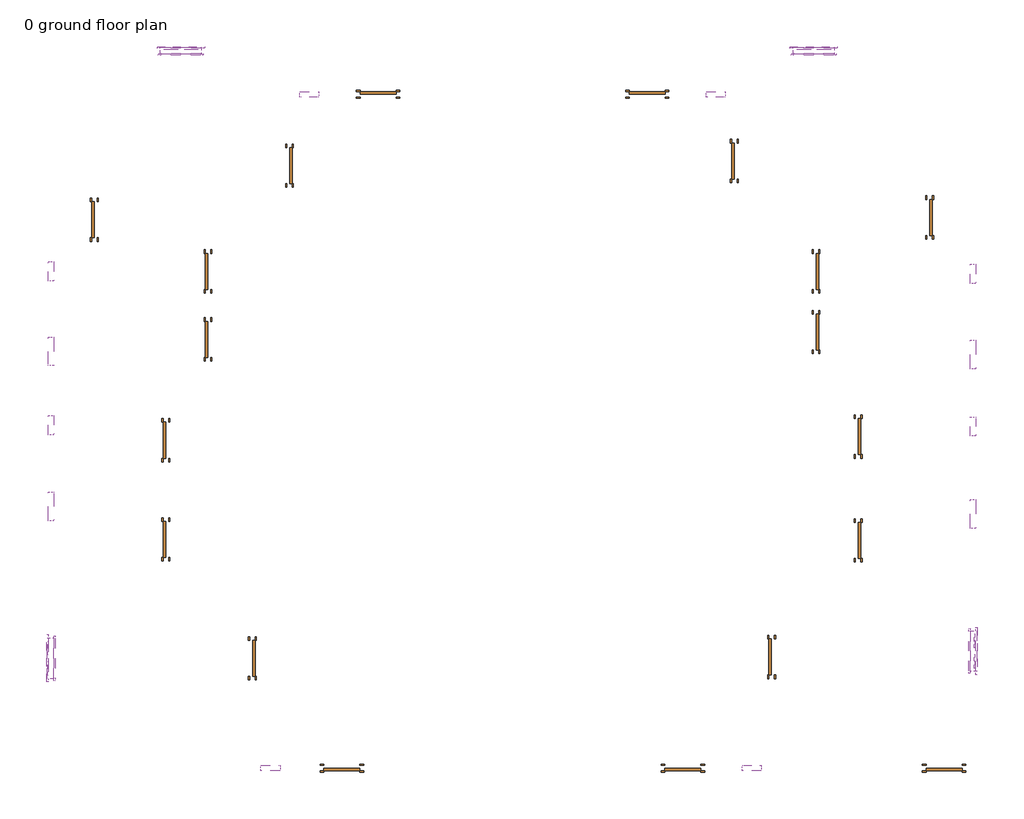
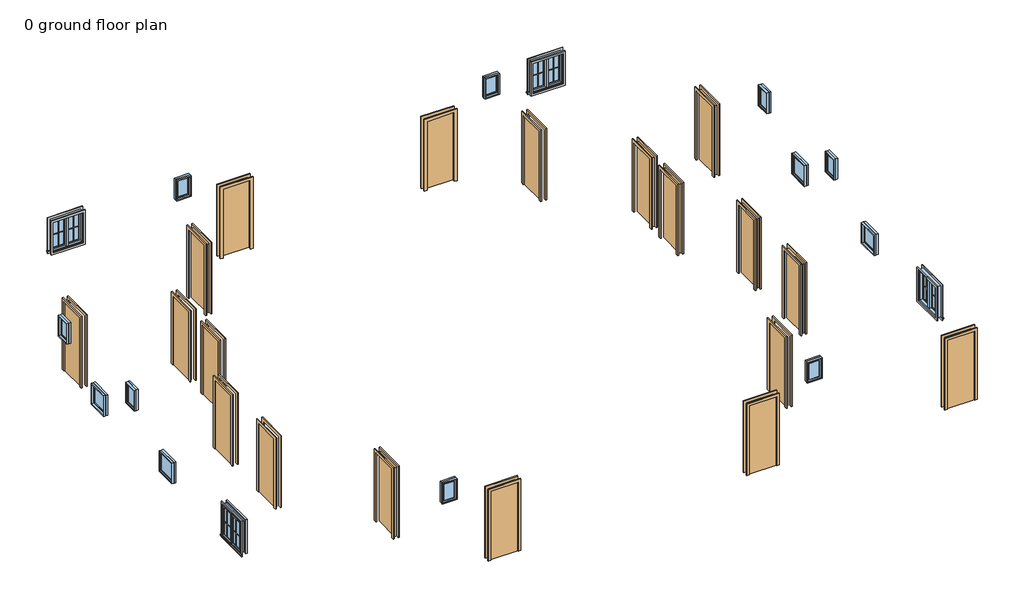
# One storey, incomplete: 19 doors, 16 proxies, 16 windows.
"""IFC4 building model written with IfcOpenShell, lengths in millimetres."""

from ifc_helpers import new_model, si_unit, origin, place, context, project, spatial, transform, mapped, element, save
from components import muntin_pattern_2x2_muntin_pattern_2x2_b3fe6957, muntin_pattern_2x2_muntin_pattern_2x2_3e0ecaf2, trim_window_exterior_flat_with_sill_41619996, trim_window_interior_flat_picture_frame_51c85655, door_f2b275c1, door_d8f5dbb5, window_a10b4202, window_0e670d86, window_a598f463

model = new_model("IFC4")

# Units and contexts
model_context = context("Model", 3, world=origin())
ifc_project = project(units=[si_unit("LENGTHUNIT", "METRE", prefix="MILLI")], contexts=[model_context])

# Site, building, storey
site = spatial("IfcSite", under=ifc_project)
building = spatial("IfcBuilding", under=site)
storey = spatial("IfcBuildingStorey", under=building, Name="0 ground floor plan", Elevation=0.0)

# Proxies
placement = place(None, origin())
muntin_pattern_2x2_muntin_pattern_2x2_shape = muntin_pattern_2x2_muntin_pattern_2x2_b3fe6957(model_context)
element("IfcBuildingElementProxy", 1, Name="Muntin Pattern_2x2 : Muntin Pattern_2x2", ObjectType="Muntin Pattern_2x2 : Muntin Pattern_2x2", at=placement, inside=storey, context=model_context, shape_type="MappedRepresentation", body=[
    mapped(muntin_pattern_2x2_muntin_pattern_2x2_shape, transform((-12267.1468188, 5178.6185601, 1593.85), x_axis=(1.0, 0.0, 0.0), y_axis=(0.0, 1.0, 0.0), z_axis=(0.0, 0.0, 1.0))),
])
element("IfcBuildingElementProxy", 2, Name="Muntin Pattern_2x2 : Muntin Pattern_2x2", ObjectType="Muntin Pattern_2x2 : Muntin Pattern_2x2", at=placement, inside=storey, context=model_context, shape_type="MappedRepresentation", body=[
    mapped(muntin_pattern_2x2_muntin_pattern_2x2_shape, transform((1105.9531812, 5178.6185601, 1593.85), x_axis=(1.0, 0.0, 0.0), y_axis=(0.0, 1.0, 0.0), z_axis=(0.0, 0.0, 1.0))),
])
element("IfcBuildingElementProxy", 3, Name="Muntin Pattern_2x2 : Muntin Pattern_2x2", ObjectType="Muntin Pattern_2x2 : Muntin Pattern_2x2", at=placement, inside=storey, context=model_context, shape_type="MappedRepresentation", body=[
    mapped(muntin_pattern_2x2_muntin_pattern_2x2_shape, transform((4733.3906812, -7341.9939399, 1593.85), x_axis=(0.0, -1.0, 0.0), y_axis=(1.0, 0.0, 0.0), z_axis=(0.0, 0.0, 1.0))),
])
element("IfcBuildingElementProxy", 4, Name="Muntin Pattern_2x2 : Muntin Pattern_2x2", ObjectType="Muntin Pattern_2x2 : Muntin Pattern_2x2", at=placement, inside=storey, context=model_context, shape_type="MappedRepresentation", body=[
    mapped(muntin_pattern_2x2_muntin_pattern_2x2_shape, transform((-14843.6593188, -7923.0189399, 1593.85), x_axis=(0.0, 1.0, 0.0), y_axis=(-1.0, 0.0, 0.0), z_axis=(0.0, 0.0, 1.0))),
])
muntin_pattern_2x2_muntin_pattern_2x2_2_shape = muntin_pattern_2x2_muntin_pattern_2x2_3e0ecaf2(model_context)
element("IfcBuildingElementProxy", 5, Name="Muntin Pattern_2x2 : Muntin Pattern_2x2", ObjectType="Muntin Pattern_2x2 : Muntin Pattern_2x2", at=placement, inside=storey, context=model_context, shape_type="MappedRepresentation", body=[
    mapped(muntin_pattern_2x2_muntin_pattern_2x2_2_shape, transform((-11838.5218188, 5178.6185601, 1593.85), x_axis=(-1.0, 0.0, 0.0), y_axis=(0.0, -1.0, 0.0), z_axis=(0.0, 0.0, 1.0))),
])
element("IfcBuildingElementProxy", 6, Name="Muntin Pattern_2x2 : Muntin Pattern_2x2", ObjectType="Muntin Pattern_2x2 : Muntin Pattern_2x2", at=placement, inside=storey, context=model_context, shape_type="MappedRepresentation", body=[
    mapped(muntin_pattern_2x2_muntin_pattern_2x2_2_shape, transform((1534.5781812, 5178.6185601, 1593.85), x_axis=(-1.0, 0.0, 0.0), y_axis=(0.0, -1.0, 0.0), z_axis=(0.0, 0.0, 1.0))),
])
element("IfcBuildingElementProxy", 7, Name="Muntin Pattern_2x2 : Muntin Pattern_2x2", ObjectType="Muntin Pattern_2x2 : Muntin Pattern_2x2", at=placement, inside=storey, context=model_context, shape_type="MappedRepresentation", body=[
    mapped(muntin_pattern_2x2_muntin_pattern_2x2_2_shape, transform((4733.3906812, -7770.6189399, 1593.85), x_axis=(0.0, 1.0, 0.0), y_axis=(-1.0, 0.0, 0.0), z_axis=(0.0, 0.0, 1.0))),
])
element("IfcBuildingElementProxy", 8, Name="Muntin Pattern_2x2 : Muntin Pattern_2x2", ObjectType="Muntin Pattern_2x2 : Muntin Pattern_2x2", at=placement, inside=storey, context=model_context, shape_type="MappedRepresentation", body=[
    mapped(muntin_pattern_2x2_muntin_pattern_2x2_2_shape, transform((-14843.6593188, -7494.3939399, 1593.85), x_axis=(0.0, -1.0, 0.0), y_axis=(1.0, 0.0, 0.0), z_axis=(0.0, 0.0, 1.0))),
])
trim_window_exterior_flat_with_sill_shape = trim_window_exterior_flat_with_sill_41619996(model_context)
element("IfcBuildingElementProxy", 9, Name="Trim-Window-Exterior-Flat : with Sill", ObjectType="Trim-Window-Exterior-Flat : with Sill", at=placement, inside=storey, context=model_context, shape_type="MappedRepresentation", body=[
    mapped(trim_window_exterior_flat_with_sill_shape, transform((-12052.8343188, 5188.1435601, 2438.4), x_axis=(-1.0, 0.0, 0.0), y_axis=(0.0, 0.0, 1.0), z_axis=(0.0, 1.0, 0.0))),
])
element("IfcBuildingElementProxy", 10, Name="Trim-Window-Exterior-Flat : with Sill", ObjectType="Trim-Window-Exterior-Flat : with Sill", at=placement, inside=storey, context=model_context, shape_type="MappedRepresentation", body=[
    mapped(trim_window_exterior_flat_with_sill_shape, transform((1320.2656812, 5188.1435601, 2438.4), x_axis=(-1.0, 0.0, 0.0), y_axis=(0.0, 0.0, 1.0), z_axis=(0.0, 1.0, 0.0))),
])
element("IfcBuildingElementProxy", 11, Name="Trim-Window-Exterior-Flat : with Sill", ObjectType="Trim-Window-Exterior-Flat : with Sill", at=placement, inside=storey, context=model_context, shape_type="MappedRepresentation", body=[
    mapped(trim_window_exterior_flat_with_sill_shape, transform((4742.9156812, -7556.3064399, 2438.4), x_axis=(0.0, 1.0, 0.0), y_axis=(0.0, 0.0, 1.0), z_axis=(1.0, 0.0, 0.0))),
])
element("IfcBuildingElementProxy", 12, Name="Trim-Window-Exterior-Flat : with Sill", ObjectType="Trim-Window-Exterior-Flat : with Sill", at=placement, inside=storey, context=model_context, shape_type="MappedRepresentation", body=[
    mapped(trim_window_exterior_flat_with_sill_shape, transform((-14853.1843188, -7708.7064399, 2438.4), x_axis=(0.0, -1.0, 0.0), y_axis=(0.0, 0.0, 1.0), z_axis=(-1.0, 0.0, 0.0))),
])
trim_window_interior_flat_picture_frame_shape = trim_window_interior_flat_picture_frame_51c85655(model_context)
element("IfcBuildingElementProxy", 13, Name="Trim-Window-Interior-Flat : Picture Frame", ObjectType="Trim-Window-Interior-Flat : Picture Frame", at=placement, inside=storey, context=model_context, shape_type="MappedRepresentation", body=[
    mapped(trim_window_interior_flat_picture_frame_shape, transform((-12052.8343188, 5073.8435601, 2438.4), x_axis=(1.0, 0.0, 0.0), y_axis=(0.0, 0.0, 1.0), z_axis=(0.0, -1.0, 0.0))),
])
element("IfcBuildingElementProxy", 14, Name="Trim-Window-Interior-Flat : Picture Frame", ObjectType="Trim-Window-Interior-Flat : Picture Frame", at=placement, inside=storey, context=model_context, shape_type="MappedRepresentation", body=[
    mapped(trim_window_interior_flat_picture_frame_shape, transform((1320.2656812, 5073.8435601, 2438.4), x_axis=(1.0, 0.0, 0.0), y_axis=(0.0, 0.0, 1.0), z_axis=(0.0, -1.0, 0.0))),
])
element("IfcBuildingElementProxy", 15, Name="Trim-Window-Interior-Flat : Picture Frame", ObjectType="Trim-Window-Interior-Flat : Picture Frame", at=placement, inside=storey, context=model_context, shape_type="MappedRepresentation", body=[
    mapped(trim_window_interior_flat_picture_frame_shape, transform((4628.6156812, -7556.3064399, 2438.4), x_axis=(0.0, -1.0, 0.0), y_axis=(0.0, 0.0, 1.0), z_axis=(-1.0, 0.0, 0.0))),
])
element("IfcBuildingElementProxy", 16, Name="Trim-Window-Interior-Flat : Picture Frame", ObjectType="Trim-Window-Interior-Flat : Picture Frame", at=placement, inside=storey, context=model_context, shape_type="MappedRepresentation", body=[
    mapped(trim_window_interior_flat_picture_frame_shape, transform((-14738.8843188, -7708.7064399, 2438.4), x_axis=(0.0, 1.0, 0.0), y_axis=(0.0, 0.0, 1.0), z_axis=(1.0, 0.0, 0.0))),
])

# Doors
door_shape = door_f2b275c1(model_context)
element("IfcDoor", 17, ObjectType="Single-Flush : 30\" x 80\"", at=placement, inside=storey, context=model_context, shape_type="MappedRepresentation", body=[
    mapped(door_shape, transform((-7885.3769874, 4216.5935601, 457.2), x_axis=(-1.0, 0.0, 0.0), y_axis=(0.0, -1.0, 0.0), z_axis=(0.0, 0.0, 1.0))),
])
element("IfcDoor", 18, ObjectType="Single-Flush : 30\" x 80\"", at=placement, inside=storey, context=model_context, shape_type="MappedRepresentation", body=[
    mapped(door_shape, transform((-13881.6343188, 1562.2935601, 457.2), x_axis=(0.0, -1.0, 0.0), y_axis=(1.0, 0.0, 0.0), z_axis=(0.0, 0.0, 1.0))),
])
element("IfcDoor", 19, ObjectType="Single-Flush : 30\" x 80\"", at=placement, inside=storey, context=model_context, shape_type="MappedRepresentation", body=[
    mapped(door_shape, transform((1371.0656812, 470.0935601, 457.2), x_axis=(0.0, 1.0, 0.0), y_axis=(-1.0, 0.0, 0.0), z_axis=(0.0, 0.0, 1.0))),
])
element("IfcDoor", 20, ObjectType="Single-Flush : 30\" x 80\"", at=placement, inside=storey, context=model_context, shape_type="MappedRepresentation", body=[
    mapped(door_shape, transform((1371.0656812, -812.6064399, 457.2), x_axis=(0.0, 1.0, 0.0), y_axis=(-1.0, 0.0, 0.0), z_axis=(0.0, 0.0, 1.0))),
])
element("IfcDoor", 21, ObjectType="Single-Flush : 30\" x 80\"", at=placement, inside=storey, context=model_context, shape_type="MappedRepresentation", body=[
    mapped(door_shape, transform((-1442.1535225, -10032.8064399, 457.2), x_axis=(1.0, 0.0, 0.0), y_axis=(0.0, 1.0, 0.0), z_axis=(0.0, 0.0, 1.0))),
])
element("IfcDoor", 22, ObjectType="Single-Flush : 30\" x 80\"", at=placement, inside=storey, context=model_context, shape_type="MappedRepresentation", body=[
    mapped(door_shape, transform((4076.1656812, -10032.8064399, 457.2), x_axis=(1.0, 0.0, 0.0), y_axis=(0.0, 1.0, 0.0), z_axis=(0.0, 0.0, 1.0))),
])
element("IfcDoor", 23, ObjectType="Single-Flush : 30\" x 80\"", at=placement, inside=storey, context=model_context, shape_type="MappedRepresentation", body=[
    mapped(door_shape, transform((-10541.5343188, -7708.7064399, 457.2), x_axis=(0.0, 1.0, 0.0), y_axis=(-1.0, 0.0, 0.0), z_axis=(0.0, 0.0, 1.0))),
])
element("IfcDoor", 24, ObjectType="Single-Flush : 30\" x 80\"", at=placement, inside=storey, context=model_context, shape_type="MappedRepresentation", body=[
    mapped(door_shape, transform((-12370.3343188, -5194.1064399, 457.2), x_axis=(0.0, -1.0, 0.0), y_axis=(1.0, 0.0, 0.0), z_axis=(0.0, 0.0, 1.0))),
])
element("IfcDoor", 25, ObjectType="Single-Flush : 30\" x 80\"", at=placement, inside=storey, context=model_context, shape_type="MappedRepresentation", body=[
    mapped(door_shape, transform((-12370.3343188, -3098.6064399, 457.2), x_axis=(0.0, -1.0, 0.0), y_axis=(1.0, 0.0, 0.0), z_axis=(0.0, 0.0, 1.0))),
])
door_2_shape = door_d8f5dbb5(model_context)
element("IfcDoor", 26, ObjectType="Single-Flush : 30\" x 80\"", at=placement, inside=storey, context=model_context, shape_type="MappedRepresentation", body=[
    mapped(door_2_shape, transform((-9758.6269874, 2705.2935601, 457.2), x_axis=(0.0, -1.0, 0.0), y_axis=(1.0, 0.0, 0.0), z_axis=(0.0, 0.0, 1.0))),
])
element("IfcDoor", 27, ObjectType="Single-Flush : 30\" x 80\"", at=placement, inside=storey, context=model_context, shape_type="MappedRepresentation", body=[
    mapped(door_2_shape, transform((-2197.6343188, 4216.5935601, 457.2), x_axis=(1.0, 0.0, 0.0), y_axis=(0.0, 1.0, 0.0), z_axis=(0.0, 0.0, 1.0))),
])
element("IfcDoor", 28, ObjectType="Single-Flush : 30\" x 80\"", at=placement, inside=storey, context=model_context, shape_type="MappedRepresentation", body=[
    mapped(door_2_shape, transform((-11481.3343188, -965.0064399, 457.2), x_axis=(0.0, 1.0, 0.0), y_axis=(-1.0, 0.0, 0.0), z_axis=(0.0, 0.0, 1.0))),
])
element("IfcDoor", 29, ObjectType="Single-Flush : 30\" x 80\"", at=placement, inside=storey, context=model_context, shape_type="MappedRepresentation", body=[
    mapped(door_2_shape, transform((-11481.3343188, 470.0935601, 457.2), x_axis=(0.0, 1.0, 0.0), y_axis=(-1.0, 0.0, 0.0), z_axis=(0.0, 0.0, 1.0))),
])
element("IfcDoor", 30, ObjectType="Single-Flush : 30\" x 80\"", at=placement, inside=storey, context=model_context, shape_type="MappedRepresentation", body=[
    mapped(door_2_shape, transform((-356.1343188, 2806.8935601, 457.2), x_axis=(0.0, 1.0, 0.0), y_axis=(-1.0, 0.0, 0.0), z_axis=(0.0, 0.0, 1.0))),
])
element("IfcDoor", 31, ObjectType="Single-Flush : 30\" x 80\"", at=placement, inside=storey, context=model_context, shape_type="MappedRepresentation", body=[
    mapped(door_2_shape, transform((3771.3656812, 1613.0935601, 457.2), x_axis=(0.0, -1.0, 0.0), y_axis=(1.0, 0.0, 0.0), z_axis=(0.0, 0.0, 1.0))),
])
element("IfcDoor", 32, ObjectType="Single-Flush : 30\" x 80\"", at=placement, inside=storey, context=model_context, shape_type="MappedRepresentation", body=[
    mapped(door_2_shape, transform((2260.0656812, -3022.4064399, 457.2), x_axis=(0.0, -1.0, 0.0), y_axis=(1.0, 0.0, 0.0), z_axis=(0.0, 0.0, 1.0))),
])
element("IfcDoor", 33, ObjectType="Single-Flush : 30\" x 80\"", at=placement, inside=storey, context=model_context, shape_type="MappedRepresentation", body=[
    mapped(door_2_shape, transform((2260.0656812, -5219.5064399, 457.2), x_axis=(0.0, -1.0, 0.0), y_axis=(1.0, 0.0, 0.0), z_axis=(0.0, 0.0, 1.0))),
])
element("IfcDoor", 34, ObjectType="Single-Flush : 30\" x 80\"", at=placement, inside=storey, context=model_context, shape_type="MappedRepresentation", body=[
    mapped(door_2_shape, transform((431.2656812, -7683.3064399, 457.2), x_axis=(0.0, 1.0, 0.0), y_axis=(-1.0, 0.0, 0.0), z_axis=(0.0, 0.0, 1.0))),
])
element("IfcDoor", 35, ObjectType="Single-Flush : 30\" x 80\"", at=placement, inside=storey, context=model_context, shape_type="MappedRepresentation", body=[
    mapped(door_2_shape, transform((-8649.2343188, -10032.8064399, 457.2), x_axis=(-1.0, 0.0, 0.0), y_axis=(0.0, -1.0, 0.0), z_axis=(0.0, 0.0, 1.0))),
])

# Windows
window_shape = window_a10b4202(model_context)
element("IfcWindow", 36, ObjectType="Fixed : 16\" x 24\"", at=placement, inside=storey, context=model_context, shape_type="MappedRepresentation", body=[
    mapped(window_shape, transform((-9299.1806531, 4216.5935601, 1651.0), x_axis=(1.0, 0.0, 0.0), y_axis=(0.0, 1.0, 0.0), z_axis=(0.0, 0.0, 1.0))),
])
element("IfcWindow", 37, ObjectType="Fixed : 16\" x 24\"", at=placement, inside=storey, context=model_context, shape_type="MappedRepresentation", body=[
    mapped(window_shape, transform((-14796.0343188, 431.9935601, 1651.0), x_axis=(0.0, -1.0, 0.0), y_axis=(1.0, 0.0, 0.0), z_axis=(0.0, 0.0, 1.0))),
])
element("IfcWindow", 38, ObjectType="Fixed : 16\" x 24\"", at=placement, inside=storey, context=model_context, shape_type="MappedRepresentation", body=[
    mapped(window_shape, transform((-14796.0343188, -2743.0064399, 1651.0), x_axis=(0.0, 1.0, 0.0), y_axis=(-1.0, 0.0, 0.0), z_axis=(0.0, 0.0, 1.0))),
])
element("IfcWindow", 39, ObjectType="Fixed : 16\" x 24\"", at=placement, inside=storey, context=model_context, shape_type="MappedRepresentation", body=[
    mapped(window_shape, transform((-10198.6343188, -10032.8064399, 1651.0), x_axis=(-1.0, 0.0, 0.0), y_axis=(0.0, -1.0, 0.0), z_axis=(0.0, 0.0, 1.0))),
])
element("IfcWindow", 40, ObjectType="Fixed : 16\" x 24\"", at=placement, inside=storey, context=model_context, shape_type="MappedRepresentation", body=[
    mapped(window_shape, transform((4685.7656812, -2768.4064399, 1651.0), x_axis=(0.0, 1.0, 0.0), y_axis=(-1.0, 0.0, 0.0), z_axis=(0.0, 0.0, 1.0))),
])
element("IfcWindow", 41, ObjectType="Fixed : 16\" x 24\"", at=placement, inside=storey, context=model_context, shape_type="MappedRepresentation", body=[
    mapped(window_shape, transform((4685.7656812, 457.3935601, 1651.0), x_axis=(0.0, 1.0, 0.0), y_axis=(-1.0, 0.0, 0.0), z_axis=(0.0, 0.0, 1.0))),
])
element("IfcWindow", 42, ObjectType="Fixed : 16\" x 24\"", at=placement, inside=storey, context=model_context, shape_type="MappedRepresentation", body=[
    mapped(window_shape, transform((-708.9201403, 4216.5935601, 1651.0), x_axis=(1.0, 0.0, 0.0), y_axis=(0.0, 1.0, 0.0), z_axis=(0.0, 0.0, 1.0))),
])
element("IfcWindow", 43, ObjectType="Fixed : 16\" x 24\"", at=placement, inside=storey, context=model_context, shape_type="MappedRepresentation", body=[
    mapped(window_shape, transform((-25.9343188, -10032.8064399, 1651.0), x_axis=(-1.0, 0.0, 0.0), y_axis=(0.0, -1.0, 0.0), z_axis=(0.0, 0.0, 1.0))),
])
window_2_shape = window_0e670d86(model_context)
element("IfcWindow", 44, ObjectType="Fixed : 24\" x 24\"", at=placement, inside=storey, context=model_context, shape_type="MappedRepresentation", body=[
    mapped(window_2_shape, transform((-14796.0343188, -1257.1064399, 609.6), x_axis=(0.0, -1.0, 0.0), y_axis=(1.0, 0.0, 0.0), z_axis=(0.0, 0.0, 1.0))),
])
element("IfcWindow", 45, ObjectType="Fixed : 24\" x 24\"", at=placement, inside=storey, context=model_context, shape_type="MappedRepresentation", body=[
    mapped(window_2_shape, transform((-14796.0343188, -4457.5064399, 609.6), x_axis=(0.0, 1.0, 0.0), y_axis=(-1.0, 0.0, 0.0), z_axis=(0.0, 0.0, 1.0))),
])
element("IfcWindow", 46, ObjectType="Fixed : 24\" x 24\"", at=placement, inside=storey, context=model_context, shape_type="MappedRepresentation", body=[
    mapped(window_2_shape, transform((4685.7656812, -1250.7564399, 609.6), x_axis=(0.0, 1.0, 0.0), y_axis=(-1.0, 0.0, 0.0), z_axis=(0.0, 0.0, 1.0))),
])
element("IfcWindow", 47, ObjectType="Fixed : 24\" x 24\"", at=placement, inside=storey, context=model_context, shape_type="MappedRepresentation", body=[
    mapped(window_2_shape, transform((4685.7656812, -4692.4564399, 609.6), x_axis=(0.0, -1.0, 0.0), y_axis=(1.0, 0.0, 0.0), z_axis=(0.0, 0.0, 1.0))),
])
window_3_shape = window_a598f463(model_context)
element("IfcWindow", 48, ObjectType="Window-Casement-Double : 34\" x 36\"", at=placement, inside=storey, context=model_context, shape_type="MappedRepresentation", body=[
    mapped(window_3_shape, transform((-12052.8343188, 5130.9935601, 609.6), x_axis=(1.0, 0.0, 0.0), y_axis=(0.0, 1.0, 0.0), z_axis=(0.0, 0.0, 1.0))),
])
element("IfcWindow", 49, ObjectType="Window-Casement-Double : 34\" x 36\"", at=placement, inside=storey, context=model_context, shape_type="MappedRepresentation", body=[
    mapped(window_3_shape, transform((1320.2656812, 5130.9935601, 609.6), x_axis=(1.0, 0.0, 0.0), y_axis=(0.0, 1.0, 0.0), z_axis=(0.0, 0.0, 1.0))),
])
element("IfcWindow", 50, ObjectType="Window-Casement-Double : 34\" x 36\"", at=placement, inside=storey, context=model_context, shape_type="MappedRepresentation", body=[
    mapped(window_3_shape, transform((4685.7656812, -7556.3064399, 609.6), x_axis=(0.0, -1.0, 0.0), y_axis=(1.0, 0.0, 0.0), z_axis=(0.0, 0.0, 1.0))),
])
element("IfcWindow", 51, ObjectType="Window-Casement-Double : 34\" x 36\"", at=placement, inside=storey, context=model_context, shape_type="MappedRepresentation", body=[
    mapped(window_3_shape, transform((-14796.0343188, -7708.7064399, 609.6), x_axis=(0.0, 1.0, 0.0), y_axis=(-1.0, 0.0, 0.0), z_axis=(0.0, 0.0, 1.0))),
])

save(model, "model.ifc")

# Revit data of these elements
# Type "Muntin Pattern_2x2 : Muntin Pattern_2x2"
#   Width [instance default] = 4' - 0"
#   Thickness = 0' - 0 1/2"
#   Height [instance default] = 4' - 0"
#   Distance = 0' - 0 3/4"
#   Interior Material [instance default] = none
#   Exterior Material [instance default] = none
#   Default Elevation = 0
# Type "Trim-Window-Exterior-Flat : with Sill"
#   Trim Width = 0' - 2 1/4"
#   Trim Thickness_Picture Frame = 0' - 1 1/4"
#   Trim Thickness_with Sill = 0' - 0 3/4"
#   Sill Thickness = 0' - 1 1/4"
#   Opening Width [instance default] = 2' - 0"
#   Opening Height [instance default] = 3' - 0"
#   Default Elevation = 4' - 0"
#   Sill = yes
#   Picture Frame = no
#   Trim Material [instance default] = none
# Type "Trim-Window-Interior-Flat : Picture Frame"
#   Trim Thickness_Picture Frame = 0' - 1 1/4"
#   Trim Width = 0' - 2 1/4"
#   Trim Thickness_with Sill = 0' - 0 3/4"
#   Sill Thickness = 0' - 1 1/4"
#   Opening Width [instance default] = 2' - 0"
#   Opening Height [instance default] = 3' - 0"
#   Default Elevation = 4' - 0"
#   Sill = no
#   Picture Frame = yes
#   Trim Material [instance default] = none
# Type "Single-Flush : 30\" x 80\""
#   Type Mark = "5"
#   Construction Type Id = "MDOOR"
#   Assembly Code = "C1020"
#   Analytic Construction = "Metal"
#   Thickness = 0' - 2"
#   Heat Transfer Coefficient (U) = 0.651978 BTU/(h·ft²·°F)
#   Height = 6' - 8"
#   Trim Projection Ext = 0' - 1"
#   Trim Projection Int = 0' - 1"
#   Trim Width = 0' - 3"
#   Width = 2' - 6"
#   Define Thermal Properties by = 1
#   Define Thermal Properties by = 1
#   Door Material = Door - Panel
#   Frame Material = Door - Frame
#   Visual Light Transmittance = 0
#   Solar Heat Gain Coefficient = 0
#   Function = (empty or 0)
#   Wall Closure = (empty or 0)
# Type "Fixed : 16\" x 24\""
#   Type Mark = "4"
#   Construction Type Id = "GSP4R"
#   Assembly Code = "B2020100"
#   Analytic Construction = "1/8 in Pilkington single glazing"
#   Visual Light Transmittance = 0.9
#   Solar Heat Gain Coefficient = 0.78
#   Heat Transfer Coefficient (U) = 0.6496 BTU/(h·ft²·°F)
#   Height = 2' - 0"
#   Default Sill Height = 3' - 0"
#   Width = 1' - 4"
#   Window Inset = 0' - 0 3/4"
#   Define Thermal Properties by = 1
#   Define Thermal Properties by = 1
#   Glass Pane Material = Glass
#   Sash Material = Sash
#   Wall Closure = (empty or 0)
# Type "Fixed : 24\" x 24\""
#   Type Mark = "3"
#   Construction Type Id = "GSP4R"
#   Assembly Code = "B2020100"
#   Analytic Construction = "1/8 in Pilkington single glazing"
#   Visual Light Transmittance = 0.9
#   Solar Heat Gain Coefficient = 0.78
#   Heat Transfer Coefficient (U) = 0.6496 BTU/(h·ft²·°F)
#   Height = 2' - 0"
#   Default Sill Height = 3' - 0"
#   Width = 2' - 0"
#   Window Inset = 0' - 0 3/4"
#   Define Thermal Properties by = 1
#   Define Thermal Properties by = 1
#   Glass Pane Material = Glass
#   Sash Material = Sash
#   Wall Closure = (empty or 0)
# Type "Window-Casement-Double : 34\" x 36\""
#   Type Mark = "14"
#   Fire Rating = "0.5h"
#   Assembly Code = "B2020100"
#   Analytic Construction = "Double glazing - domestic"
#   Frame Extension [instance default] = 0' - 0 1/4"
#   Window Inset [instance default] = 0' - 0"
#   Wall Thickness [instance default] = 0' - 6"
#   Interior Wall Closure [instance default] = 0' - 2 1/4"
#   Half Width = 1' - 5"
#   Visual Light Transmittance = 0.81
#   Thermal Resistance (R) = 1.8146 (h·ft²·°F)/BTU
#   Solar Heat Gain Coefficient = 0.76
#   Rough Width = 2' - 10 1/2"
#   Rough Height = 3' - 0 1/2"
#   Height = 3' - 0"
#   Heat Transfer Coefficient (U) = 0.5511 BTU/(h·ft²·°F)
#   Exterior Wall Closure [instance default] = 0' - 1 1/4"
#   Extension Jamb [instance default] = 0' - 2 1/4"
#   Default Sill Height = 3' - 0"
#   Width = 2' - 10"
#   Define Thermal Properties by = 0
#   Muntin Visibility = yes
#   Interior Trim Visibility [instance default] = yes
#   Exterior Trim Visibility [instance default] = yes
#   Extension Jamb Visibility [instance default] = yes
#   Interior Trim Material = Wood - Stained
#   Muntin Pattern = Muntin Pattern_2x2 : Muntin Pattern_2x2
#   Interior Trim = Trim-Window-Interior-Flat : Picture Frame
#   Interior Frame Material = Wood - Stained
#   Glass Panel Material = Glass
#   Exterior Trim Material = Clad - White
#   Exterior Trim = Trim-Window-Exterior-Flat : with Sill
#   Exterior Frame Material = Clad - White
#   Wall Closure = (empty or 0)
# Elements 1, 2, 3, 4, 5, 6, 7, 8 (IfcBuildingElementProxy, "Muntin Pattern_2x2 : Muntin Pattern_2x2")
#   Width = 0' - 11 5/8"
#   Height = 2' - 6 1/2"
#   Interior Material = Wood - Stained
#   Exterior Material = Clad - White
#   Phase Created = New Construction
#   Materials on its faces: "Clad - White", "Wood - Stained"
# Elements 9, 10, 11, 12 (IfcBuildingElementProxy, "Trim-Window-Exterior-Flat : with Sill")
#   Opening Width = 2' - 10"
#   Opening Height = 3' - 0"
#   Trim Material = Clad - White
#   Phase Created = New Construction
#   Materials on its faces: "Clad - White"
# Elements 13, 14, 15, 16 (IfcBuildingElementProxy, "Trim-Window-Interior-Flat : Picture Frame")
#   Opening Width = 2' - 10"
#   Opening Height = 3' - 0"
#   Trim Material = Wood - Stained
#   Phase Created = New Construction
#   Materials on its faces: "Wood - Stained"
# Elements 17, 18, 19, 20, 21, 22, 23, 24, 25, 26, 27, 28, 29, 30, 31, 32, 33, 34, 35 (IfcDoor, "Single-Flush : 30\" x 80\"")
#   Phase Created = New Construction
#   Materials on its faces: "Door - Frame", "Door - Panel"
# Element 36 (IfcWindow, "Fixed : 16\" x 24\"")
#   Mark = "5"
#   Phase Created = New Construction
#   Materials on its faces: "Sash", "Glass"
# Element 37 (IfcWindow, "Fixed : 16\" x 24\"")
#   Mark = "6"
#   Phase Created = New Construction
#   Materials on its faces: "Sash", "Glass"
# Element 38 (IfcWindow, "Fixed : 16\" x 24\"")
#   Mark = "7"
#   Phase Created = New Construction
#   Materials on its faces: "Sash", "Glass"
# Element 39 (IfcWindow, "Fixed : 16\" x 24\"")
#   Mark = "8"
#   Phase Created = New Construction
#   Materials on its faces: "Sash", "Glass"
# Element 40 (IfcWindow, "Fixed : 16\" x 24\"")
#   Mark = "9"
#   Phase Created = New Construction
#   Materials on its faces: "Sash", "Glass"
# Element 41 (IfcWindow, "Fixed : 16\" x 24\"")
#   Mark = "10"
#   Phase Created = New Construction
#   Materials on its faces: "Sash", "Glass"
# Element 42 (IfcWindow, "Fixed : 16\" x 24\"")
#   Mark = "11"
#   Phase Created = New Construction
#   Materials on its faces: "Sash", "Glass"
# Element 43 (IfcWindow, "Fixed : 16\" x 24\"")
#   Mark = "20"
#   Phase Created = New Construction
#   Materials on its faces: "Sash", "Glass"
# Element 44 (IfcWindow, "Fixed : 24\" x 24\"")
#   Mark = "16"
#   Phase Created = New Construction
#   Materials on its faces: "Sash", "Glass"
# Element 45 (IfcWindow, "Fixed : 24\" x 24\"")
#   Mark = "17"
#   Phase Created = New Construction
#   Materials on its faces: "Sash", "Glass"
# Element 46 (IfcWindow, "Fixed : 24\" x 24\"")
#   Mark = "18"
#   Phase Created = New Construction
#   Materials on its faces: "Sash", "Glass"
# Element 47 (IfcWindow, "Fixed : 24\" x 24\"")
#   Mark = "19"
#   Phase Created = New Construction
#   Materials on its faces: "Sash", "Glass"
# Element 48 (IfcWindow, "Window-Casement-Double : 34\" x 36\"")
#   Mark = "1"
#   Window Inset = 0' - 0"
#   Interior Wall Closure = 0' - 2 1/4"
#   Frame Extension = 0' - 0 1/4"
#   Exterior Wall Closure = 0' - 1 1/4"
#   Interior Trim Visibility = yes
#   Exterior Trim Visibility = yes
#   Phase Created = New Construction
#   Materials on its faces: "Wood - Stained", "Glass", "Clad - White"
# Element 49 (IfcWindow, "Window-Casement-Double : 34\" x 36\"")
#   Mark = "2"
#   Window Inset = 0' - 0"
#   Interior Wall Closure = 0' - 2 1/4"
#   Frame Extension = 0' - 0 1/4"
#   Exterior Wall Closure = 0' - 1 1/4"
#   Interior Trim Visibility = yes
#   Exterior Trim Visibility = yes
#   Phase Created = New Construction
#   Materials on its faces: "Wood - Stained", "Glass", "Clad - White"
# Element 50 (IfcWindow, "Window-Casement-Double : 34\" x 36\"")
#   Mark = "3"
#   Window Inset = 0' - 0"
#   Interior Wall Closure = 0' - 2 1/4"
#   Frame Extension = 0' - 0 1/4"
#   Exterior Wall Closure = 0' - 1 1/4"
#   Interior Trim Visibility = yes
#   Exterior Trim Visibility = yes
#   Phase Created = New Construction
#   Materials on its faces: "Wood - Stained", "Glass", "Clad - White"
# Element 51 (IfcWindow, "Window-Casement-Double : 34\" x 36\"")
#   Mark = "4"
#   Window Inset = 0' - 0"
#   Interior Wall Closure = 0' - 2 1/4"
#   Frame Extension = 0' - 0 1/4"
#   Exterior Wall Closure = 0' - 1 1/4"
#   Interior Trim Visibility = yes
#   Exterior Trim Visibility = yes
#   Phase Created = New Construction
#   Materials on its faces: "Wood - Stained", "Glass", "Clad - White"
# Materials
#   "Door - Panel": class "Wood", colour RGB 210 159 95, transparency 0, Cost = 0
#   "Door - Frame": colour RGB 118 70 51, transparency 0, Cost = 0
#   "Glass": class "Glass", colour RGB 0 128 192, transparency 0.75, Description = "Soda Lime Glass", Cost = 0
#   "Sash": class "Wood", colour RGB 224 178 126, transparency 0, Cost = 0
#   "Wood - Stained": class "Wood", colour RGB 224 178 126, transparency 0, Cost = 0
#   "Clad - White": class "Wood", colour RGB 242 242 238, transparency 0, Cost = 0
